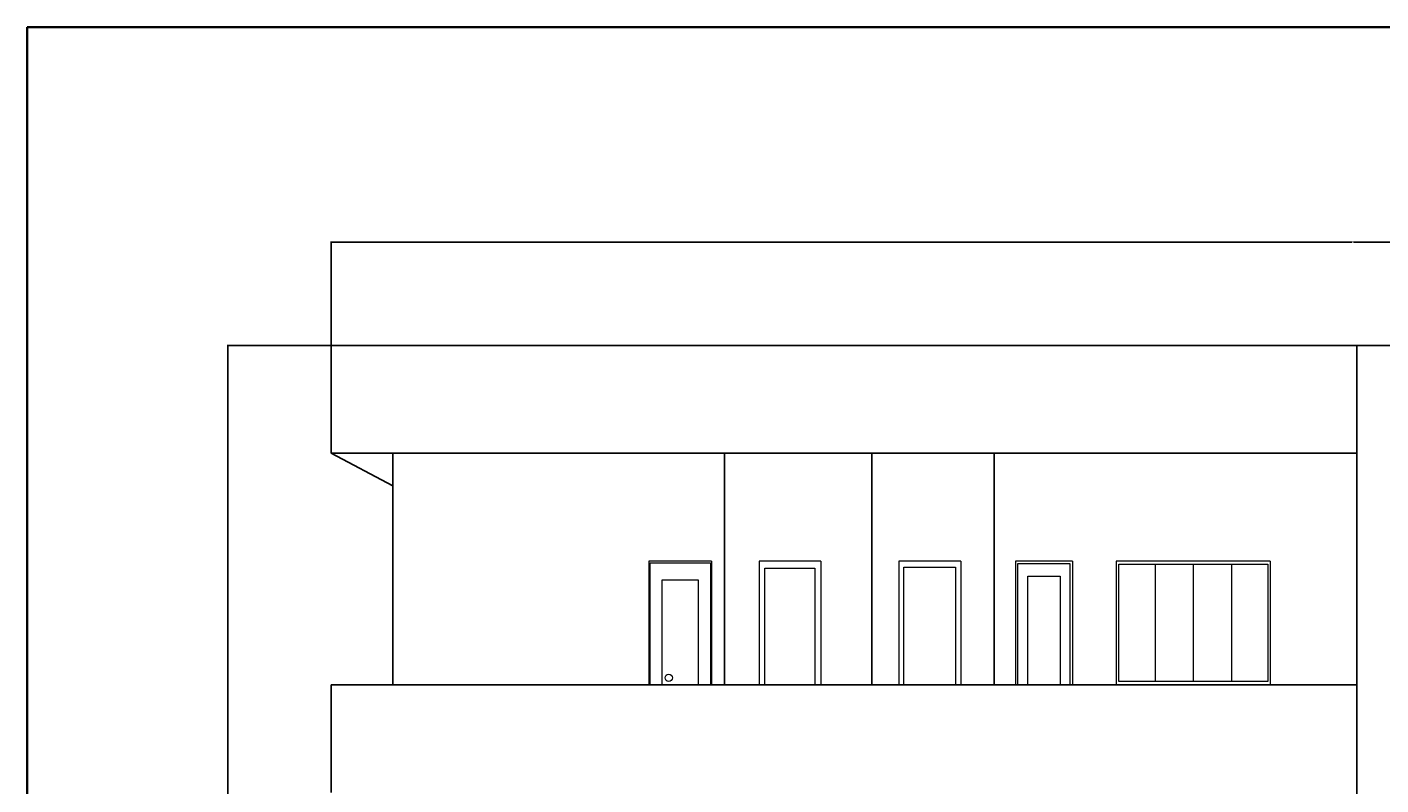
# Model space of a CAD drawing. Units: inches. Extents: x 2120 to 4013, y 1390 to 3019.
# Tile 48 of 59: x 2120 to 2647, y 2724 to 3019. Entities that reach past the tile are written whole.
import ezdxf

# ---------------------------------------------------------------- set-up
doc = ezdxf.new("R2010")
doc.units = ezdxf.units.IN
for name, color, linetype, lineweight in [('A-ANNO-DIMS', 2, 'Continuous', 18), ('A-ANNO-TTLB', 7, 'Continuous', 35), ('A-DOOR', 3, 'Continuous', 18), ('A-ELEV', 7, 'Continuous', 25), ('A-GLAZ', 4, 'Continuous', 18)]:
    doc.layers.add(name, color=color, linetype=linetype, lineweight=lineweight)
doc.styles.get("Standard").update_dxf_attribs({"font": 'arial.ttf'})
doc.dimstyles.get("Standard").update_dxf_attribs({"dimtxt": 0.18, "dimasz": 0.18, "dimexe": 0.18, "dimexo": 0.0625, "dimgap": 0.09, "dimtad": 0, "dimtih": 1, "dimtoh": 1, "dimdec": 4, "dimzin": 0, "dimdsep": 46, "dimtxsty": 'Standard', "dimcen": 0.09, "dimadec": 0, "dimazin": 0, "dimtfac": 1, "dimtdec": 4, "dimtofl": 0, "dimtmove": 0, "dimatfit": 3, "dimfxl": 1, "dimtolj": 1, "dimtzin": 0, "dimarcsym": 0})

# ---------------------------------------------------------------- blocks, each defined once
blk = doc.blocks.new('*D223')
at = {"layer": 'A-ANNO-DIMS', "color": 0, "lineweight": -2, "transparency": 16777216}
for p, q in [((2238.73, 2895.37), (2238.73, 2935.69)), ((2238.91, 2935.51), (2635.94, 2935.51)), ((3033.55, 2935.51), (2636.52, 2935.51)), ((3033.73, 2895.37), (3033.73, 2935.69))]:
    blk.add_line(p, q, dxfattribs=at)
at = {"layer": 'A-ANNO-DIMS', "color": 0, "transparency": 16777216}
for points in [[(2238.91, 2935.54), (2238.91, 2935.48), (2238.73, 2935.51)], [(3033.55, 2935.54), (3033.55, 2935.48), (3033.73, 2935.51)]]:
    blk.add_solid(points, dxfattribs=at)
at = {"layer": 'Defpoints', "color": 0, "transparency": 16777216}
for p in [(3033.73, 2935.51), (2238.73, 2895.31), (3033.73, 2895.31)]:
    blk.add_point(p, dxfattribs=at)
at = {"layer": 'A-ANNO-DIMS', "color": 0, "transparency": 16777216, "insert": (2636.23, 2935.51), "char_height": 0.18, "attachment_point": 5}
blk.add_mtext('\\A1;795', dxfattribs=at)
blk = doc.blocks.new('*D224')
at = {"layer": 'A-ANNO-DIMS', "color": 0, "lineweight": -2, "transparency": 16777216}
for p, q in [((2238.67, 2895.31), (2198.35, 2895.31)), ((2198.53, 2895.13), (2198.53, 2682.49)), ((2198.53, 2469.49), (2198.53, 2682.13)), ((2262.67, 2469.31), (2198.35, 2469.31))]:
    blk.add_line(p, q, dxfattribs=at)
at = {"layer": 'A-ANNO-DIMS', "color": 0, "transparency": 16777216}
for points in [[(2198.5, 2895.13), (2198.56, 2895.13), (2198.53, 2895.31)], [(2198.5, 2469.49), (2198.56, 2469.49), (2198.53, 2469.31)]]:
    blk.add_solid(points, dxfattribs=at)
at = {"layer": 'Defpoints', "color": 0, "transparency": 16777216}
for p in [(2198.53, 2895.31), (2238.73, 2895.31), (2262.73, 2469.31)]:
    blk.add_point(p, dxfattribs=at)
at = {"layer": 'A-ANNO-DIMS', "color": 0, "transparency": 16777216, "insert": (2198.53, 2682.31), "char_height": 0.18, "attachment_point": 5}
blk.add_mtext('\\A1;426', dxfattribs=at)

msp = doc.modelspace()

# ---------------------------------------------------------------- linework, layer by layer
at = {"layer": 'A-ANNO-TTLB'}
msp.add_lwpolyline([(2120.4581, 3019.1237), (4012.9334, 3019.1237), (4012.9334, 1390.2222), (2120.4581, 1390.2222)], close=True, dxfattribs=at)
at = {"layer": 'A-DOOR'}
for p, q in [((2362.3957, 2811.3118), (2362.3957, 2763.3118)), ((2386.7425, 2811.3118), (2362.3957, 2811.3118)), ((2362.3957, 2811.3118), (2362.3957, 2763.3118)), ((2386.7425, 2811.3118), (2362.3957, 2811.3118)), ((2386.7425, 2811.3118), (2386.7425, 2763.3118)), ((2386.7425, 2811.3118), (2386.7425, 2763.3118)), ((2505.0196, 2811.3118), (2505.0196, 2763.3118)), ((2527.1368, 2811.3118), (2505.0196, 2811.3118)), ((2505.0196, 2811.3118), (2505.0196, 2763.3118)), ((2527.1368, 2811.3118), (2505.0196, 2811.3118)), ((2527.1368, 2811.3118), (2527.1368, 2763.3118)), ((2527.1368, 2811.3118), (2527.1368, 2763.3118))]:
    msp.add_line(p, q, dxfattribs=at)
for points in [[(2362.8987, 2763.3118), (2362.8987, 2810.6544), (2386.362, 2810.6544), (2386.362, 2763.3118)], [(2505.9355, 2763.3118), (2505.9355, 2810.4713), (2526.1603, 2810.4713), (2526.1603, 2763.3118)], [(2367.5645, 2763.3118), (2367.5645, 2804.0397), (2381.4937, 2804.0397), (2381.4937, 2763.3118)], [(2509.792, 2763.3118), (2509.792, 2805.4761), (2522.4068, 2805.4761), (2522.4068, 2763.3118)]]:
    msp.add_lwpolyline(points, dxfattribs=at)
msp.add_circle((2370.0892, 2765.9453), 1.423, dxfattribs=at)
at = {"layer": 'A-ELEV'}
for p, q in [((2238.7331, 2853.3118), (2238.7331, 2895.3118)), ((2637.7331, 2895.3118), (2238.7331, 2895.3118)), ((2637.7331, 2895.3118), (2637.7331, 2727.3118)), ((2637.7331, 2895.3118), (2715.7331, 2895.3118)), ((2637.7331, 2853.3118), (2238.7331, 2853.3118)), ((2238.7331, 2853.3118), (2262.7331, 2840.6916)), ((2262.7331, 2853.3118), (2262.7331, 2763.3118)), ((2391.7331, 2853.3118), (2391.7331, 2763.3118)), ((2449.0524, 2853.3118), (2449.0524, 2763.3118)), ((2496.7331, 2763.3118), (2496.7331, 2853.3118)), ((2262.7331, 2769.3118), (2262.7331, 2763.3118)), ((2238.7331, 2721.3118), (2238.7331, 2763.3118)), ((2637.7331, 2763.3118), (2238.7331, 2763.3118)), ((2238.7331, 2763.3118), (2238.7331, 2721.3118)), ((2637.7331, 2763.3118), (2637.7331, 2601.3118))]:
    msp.add_line(p, q, dxfattribs=at)
at = {"layer": 'A-GLAZ'}
for p, q in [((2405.3032, 2811.3118), (2405.3032, 2763.3118)), ((2429.3032, 2811.3118), (2405.3032, 2811.3118)), ((2405.3032, 2811.3118), (2405.3032, 2763.3118)), ((2429.3032, 2811.3118), (2405.3032, 2811.3118)), ((2429.3032, 2811.3118), (2429.3032, 2763.3118)), ((2429.3032, 2811.3118), (2429.3032, 2763.3118)), ((2459.6703, 2811.3118), (2459.6703, 2763.3118)), ((2483.6703, 2811.3118), (2459.6703, 2811.3118)), ((2459.6703, 2811.3118), (2459.6703, 2763.3118)), ((2483.6703, 2811.3118), (2459.6703, 2811.3118)), ((2483.6703, 2811.3118), (2483.6703, 2763.3118)), ((2483.6703, 2811.3118), (2483.6703, 2763.3118)), ((2544.1361, 2811.3118), (2544.1361, 2763.3118)), ((2604.1361, 2811.3118), (2544.1361, 2811.3118)), ((2544.1361, 2811.3118), (2544.1361, 2763.3118)), ((2604.1361, 2811.3118), (2544.1361, 2811.3118)), ((2559.2822, 2810.2237), (2559.2822, 2764.4997)), ((2574.1465, 2810.2237), (2574.1465, 2764.4997)), ((2589.0012, 2810.2237), (2589.0012, 2764.4997)), ((2604.1361, 2811.3118), (2604.1361, 2763.3118)), ((2604.1361, 2811.3118), (2604.1361, 2763.3118)), ((2429.3032, 2763.3118), (2405.3032, 2763.3118)), ((2429.3032, 2763.3118), (2405.3032, 2763.3118)), ((2483.6703, 2763.3118), (2459.6703, 2763.3118)), ((2483.6703, 2763.3118), (2459.6703, 2763.3118)), ((2604.1361, 2763.3118), (2544.1361, 2763.3118)), ((2604.1361, 2763.3118), (2544.1361, 2763.3118))]:
    msp.add_line(p, q, dxfattribs=at)
for points in [[(2407.4945, 2763.3118), (2407.4945, 2808.6586), (2426.8868, 2808.6586), (2426.8868, 2763.3118)], [(2461.5996, 2763.3118), (2461.5996, 2808.9767), (2481.6066, 2808.9767), (2481.6066, 2763.3118)]]:
    msp.add_lwpolyline(points, dxfattribs=at)
msp.add_lwpolyline([(2545.1381, 2810.2237), (2603.1548, 2810.2237), (2603.1548, 2764.4997), (2545.1381, 2764.4997)], close=True, dxfattribs=at)

# ---------------------------------------------------------------- dimensions: what is measured, and where the dimension line sits
at = {"layer": 'A-ANNO-DIMS'}
dim = msp.add_linear_dim(base=(3033.7331, 2935.5118), p1=(2238.7331, 2895.3118), p2=(3033.7331, 2895.3118), dimstyle='Standard', override={"dimdec": 0, "dimlfac": 1, "dimrnd": 0, "dimzin": 0, "dimdsep": 46, "dimlunit": 2}, dxfattribs=at)
dim.commit()
dim.dimension.update_dxf_attribs({"geometry": '*D223', "text_midpoint": (2636.2331, 2935.5118)})
dim = msp.add_linear_dim(base=(2198.5331, 2895.3118), p1=(2262.7331, 2469.3118), p2=(2238.7331, 2895.3118), angle=90, dimstyle='Standard', override={"dimdec": 0, "dimlfac": 1, "dimrnd": 0, "dimzin": 0, "dimdsep": 46, "dimlunit": 2}, dxfattribs=at)
dim.commit()
dim.dimension.update_dxf_attribs({"geometry": '*D224', "text_midpoint": (2198.5331, 2682.3118)})

doc.saveas('drawing.dxf')
